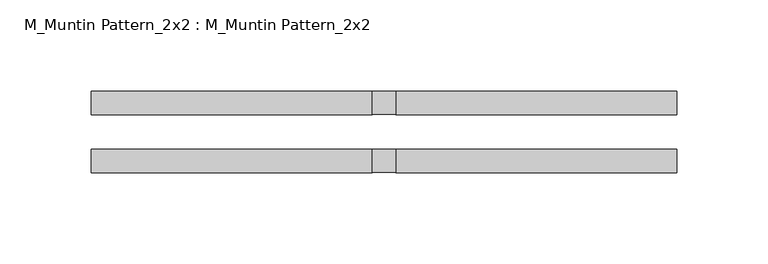
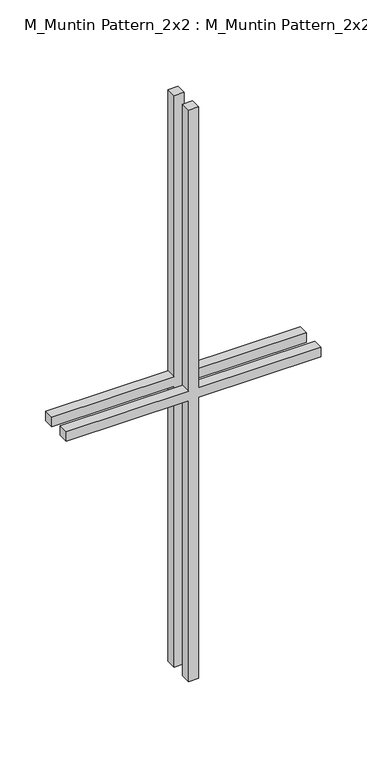
"""IFC4 building model written with IfcOpenShell, lengths in millimetres: proxy geometry, M_Muntin Pattern_2x2 : M_Muntin Pattern_2x2."""

from ifc_helpers import new_model, si_unit, frame, origin, place, context, project, spatial, polyline, outline, extrude, source, transform, mapped, element, save


def m_muntin_pattern_2x2_m_muntin_pattern_2x2_a9b7b7a9(model_context):
    return source(origin(), model_context, "Body", "SweptSolid", [
        extrude(outline(polyline([(386.5, -6.35), (386.5, -160.3375), (373.8, -160.3375), (373.8, -6.35), (0.0, -6.35), (0.0, 6.35), (373.8, 6.35), (373.8, 160.3375), (386.5, 160.3375), (386.5, 6.35), (760.3, 6.35), (760.3, -6.35), (386.5, -6.35)])), frame((0.0, -22.225, 0.0), z_axis=(0.0, 1.0, 0.0), x_axis=(0.0, 0.0, 1.0)), (0.0, 0.0, 1.0), 12.7),
        extrude(outline(polyline([(386.5, -6.35), (386.5, -160.3375), (373.8, -160.3375), (373.8, -6.35), (0.0, -6.35), (0.0, 6.35), (373.8, 6.35), (373.8, 160.3375), (386.5, 160.3375), (386.5, 6.35), (760.3, 6.35), (760.3, -6.35), (386.5, -6.35)])), frame((0.0, 9.525, 0.0), z_axis=(0.0, 1.0, 0.0), x_axis=(0.0, 0.0, 1.0)), (0.0, 0.0, 1.0), 12.7),
    ])


if __name__ == "__main__":
    model = new_model("IFC4")
    model_context = context("Model", 3, world=origin())
    ifc_project = project(units=[si_unit("LENGTHUNIT", "METRE", prefix="MILLI")], contexts=[model_context])
    site = spatial("IfcSite", under=ifc_project)
    building = spatial("IfcBuilding", under=site)
    placement = place(None, origin())
    m_muntin_pattern_2x2_m_muntin_pattern_2x2_shape = m_muntin_pattern_2x2_m_muntin_pattern_2x2_a9b7b7a9(model_context)
    element("IfcBuildingElementProxy", 1, Name="M_Muntin Pattern_2x2 : M_Muntin Pattern_2x2", ObjectType="M_Muntin Pattern_2x2 : M_Muntin Pattern_2x2", at=placement, inside=building, context=model_context, shape_type="MappedRepresentation", body=[
        mapped(m_muntin_pattern_2x2_m_muntin_pattern_2x2_shape, transform((0.0, 0.0, 0.0), x_axis=(1.0, 0.0, 0.0), y_axis=(0.0, 1.0, 0.0), z_axis=(0.0, 0.0, 1.0))),
    ])
    save(model, "model.ifc")

# Revit data of these elements
# Type "M_Muntin Pattern_2x2 : M_Muntin Pattern_2x2"
#   Width [instance default] = 3' - 11.24409"
#   Thickness = 0' - 0 1/2"
#   Height [instance default] = 3' - 11.24409"
#   Distance = 0' - 0 3/4"
#   Interior Material [instance default] = none
#   Exterior Material [instance default] = none
#   Default Elevation = 0
# Element 1 (IfcBuildingElementProxy, "M_Muntin Pattern_2x2 : M_Muntin Pattern_2x2")
#   Width = 1' - 0 5/8"
#   Height = 2' - 5.93307"
#   Interior Material = Wood - Stained
#   Exterior Material = Clad - White
#   Materials on its faces: "Clad - White", "Wood - Stained"
# Materials
#   "Clad - White": class "Wood", colour RGB 242 242 238, transparency 0, Cost = 0
#   "Wood - Stained": class "Wood", colour RGB 227 170 128, transparency 0, Cost = 0
